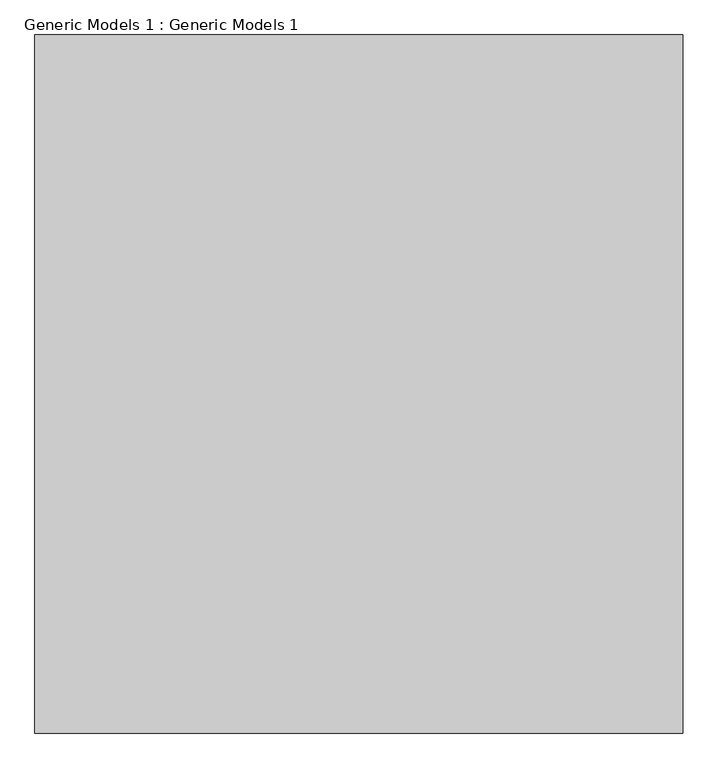
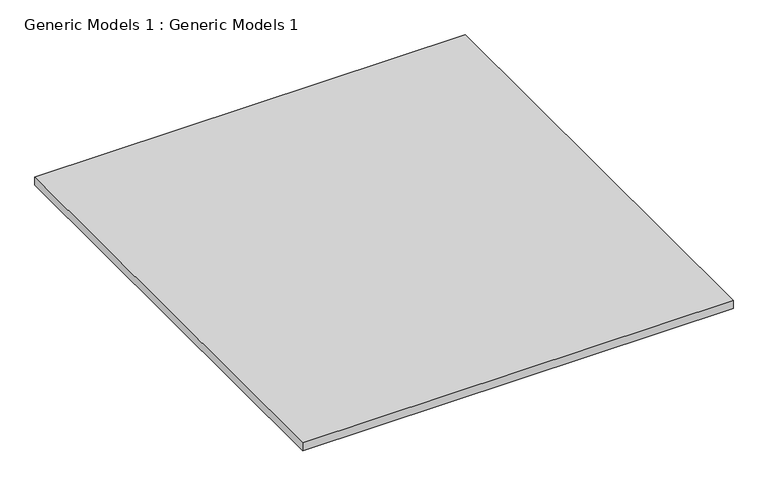
"""IFC4 building model written with IfcOpenShell, lengths in millimetres: proxy geometry, Generic Models 1 : Generic Models 1."""

from ifc_helpers import new_model, si_unit, frame, origin, place, context, project, spatial, polyline, outline, extrude, source, transform, mapped, element, save


def generic_models_1_generic_models_1_92ce0f77(model_context):
    return source(origin(), model_context, "Body", "SweptSolid", [
        extrude(outline(polyline([(-6340.991855, 1454.1639573), (-6340.991855, -15759.1538163), (-22327.6806893, -15759.1538163), (-22327.6806893, 1454.1639573), (-6340.991855, 1454.1639573)])), frame((0.0, 0.0, -304.8), z_axis=(0.0, 0.0, 1.0), x_axis=(1.0, 0.0, 0.0)), (0.0, 0.0, 1.0), 304.8),
    ])


if __name__ == "__main__":
    model = new_model("IFC4")
    model_context = context("Model", 3, world=origin())
    ifc_project = project(units=[si_unit("LENGTHUNIT", "METRE", prefix="MILLI")], contexts=[model_context])
    site = spatial("IfcSite", under=ifc_project)
    building = spatial("IfcBuilding", under=site)
    placement = place(None, origin())
    generic_models_1_generic_models_1_shape = generic_models_1_generic_models_1_92ce0f77(model_context)
    element("IfcBuildingElementProxy", 1, Name="Generic Models 1 : Generic Models 1", ObjectType="Generic Models 1 : Generic Models 1", at=placement, inside=building, context=model_context, shape_type="MappedRepresentation", body=[
        mapped(generic_models_1_generic_models_1_shape, transform((0.0, 0.0, 0.0), x_axis=(1.0, 0.0, 0.0), y_axis=(0.0, 1.0, 0.0), z_axis=(0.0, 0.0, 1.0))),
    ])
    save(model, "model.ifc")
